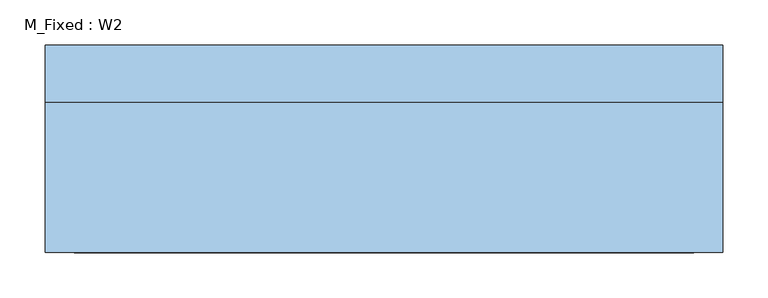
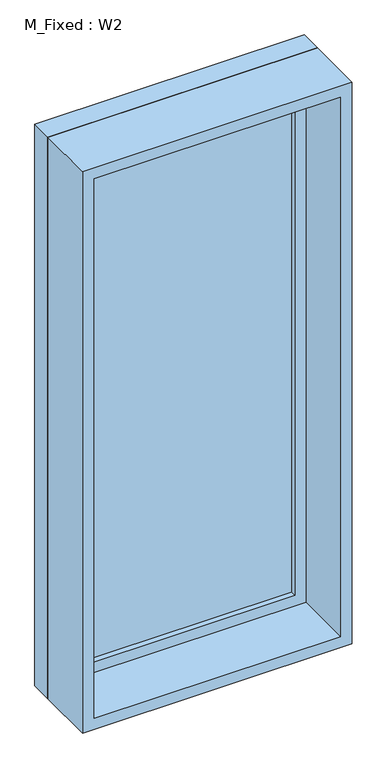
"""IFC4 building model written with IfcOpenShell, lengths in millimetres: window geometry, M_Fixed : W2."""

from ifc_helpers import new_model, si_unit, frame, origin, place, context, project, spatial, polyline, outline, extrude, source, transform, mapped, element, save


def m_fixed_w2_a119b0d1(model_context):
    return source(origin(), model_context, "Body", "SweptSolid", [
        extrude(outline(polyline([(-312.0, 93.0), (312.0, 93.0), (312.0, 81.0), (-312.0, 81.0), (-312.0, 93.0)])), frame((0.0, 0.0, 513.0), z_axis=(0.0, 0.0, 1.0), x_axis=(1.0, 0.0, 0.0)), (0.0, 0.0, 1.0), 1524.0),
        extrude(outline(polyline([(2081.0, -356.0), (469.0, -356.0), (469.0, 356.0), (2081.0, 356.0), (2081.0, -356.0)]), holes=[polyline([(2037.0, -312.0), (2037.0, 312.0), (513.0, 312.0), (513.0, -312.0), (2037.0, -312.0)])]), frame((0.0, 65.0, 0.0), z_axis=(0.0, 1.0, 0.0), x_axis=(0.0, 0.0, 1.0)), (0.0, 0.0, 1.0), 44.0),
        extrude(outline(polyline([(2100.0, -375.0), (450.0, -375.0), (450.0, 375.0), (2100.0, 375.0), (2100.0, -375.0)]), holes=[polyline([(2081.0, -356.0), (2081.0, 356.0), (469.0, 356.0), (469.0, -356.0), (2081.0, -356.0)])]), frame((0.0, 65.0, 0.0), z_axis=(0.0, 1.0, 0.0), x_axis=(0.0, 0.0, 1.0)), (0.0, 0.0, 1.0), 63.0),
        extrude(outline(polyline([(2100.0, -375.0), (450.0, -375.0), (450.0, 375.0), (2100.0, 375.0), (2100.0, -375.0)]), holes=[polyline([(2068.0, -343.0), (2068.0, 343.0), (482.0, 343.0), (482.0, -343.0), (2068.0, -343.0)])]), frame((0.0, -102.0, 0.0), z_axis=(0.0, 1.0, 0.0), x_axis=(0.0, 0.0, 1.0)), (0.0, 0.0, 1.0), 167.0),
    ])


if __name__ == "__main__":
    model = new_model("IFC4")
    model_context = context("Model", 3, world=origin())
    ifc_project = project(units=[si_unit("LENGTHUNIT", "METRE", prefix="MILLI")], contexts=[model_context])
    site = spatial("IfcSite", under=ifc_project)
    building = spatial("IfcBuilding", under=site)
    placement = place(None, origin())
    m_fixed_w2_shape = m_fixed_w2_a119b0d1(model_context)
    element("IfcWindow", 1, ObjectType="M_Fixed : W2", at=placement, inside=building, context=model_context, shape_type="MappedRepresentation", body=[
        mapped(m_fixed_w2_shape, transform((0.0, 0.0, 0.0), x_axis=(1.0, 0.0, 0.0), y_axis=(0.0, 1.0, 0.0), z_axis=(0.0, 0.0, 1.0))),
    ])
    save(model, "model.ifc")

# Revit data of these elements
# Type "M_Fixed : W2"
#   Type Mark = "20"
#   Height = 1650 mm
#   Default Sill Height = 450 mm
#   Width = 750 mm
#   Window Inset = 19 mm
#   Frame Exterior Material = Iron, Ductile
#   Frame Interior Material = Iron, Ductile
#   Glass Pane Material = Glass
#   Sash = Iron, Ductile
#   Wall Closure = (empty or 0)
# Element 1 (IfcWindow, "M_Fixed : W2")
#   Materials on its faces: "Iron, Ductile", "Glass"
# Materials
#   "Iron, Ductile": class "Metal", colour RGB 90 97 102, transparency 0, Description = "Ductile cast iron", Cost = 0
#   "Glass": class "Glass", colour RGB 218 227 224, transparency 0.85, Description = "Soda Lime Glass", Cost = 0
